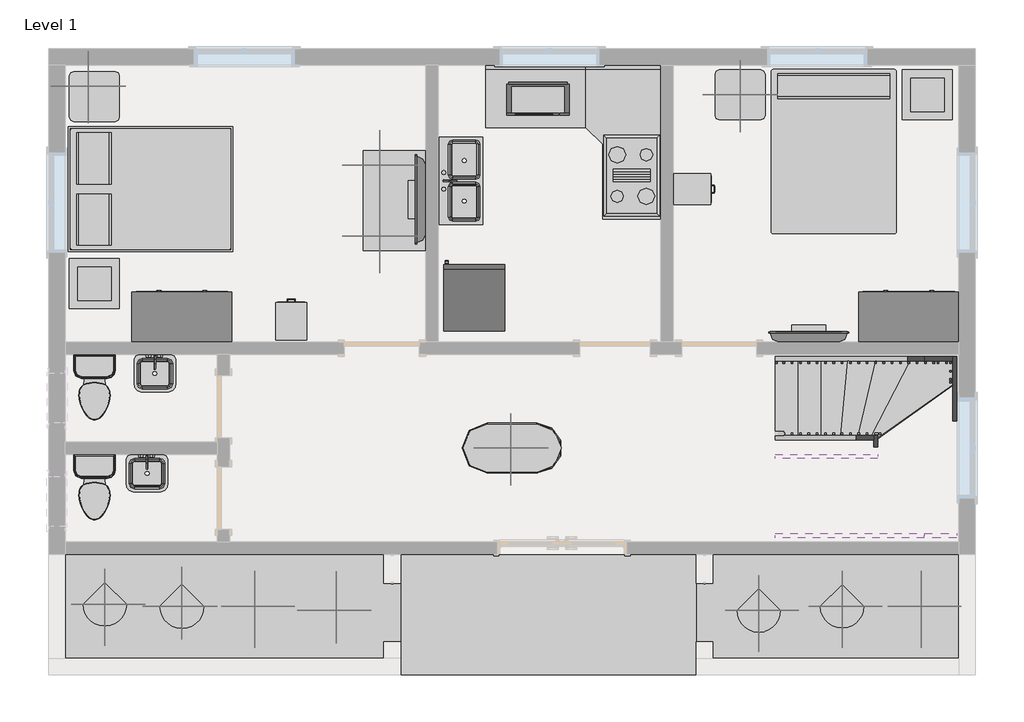
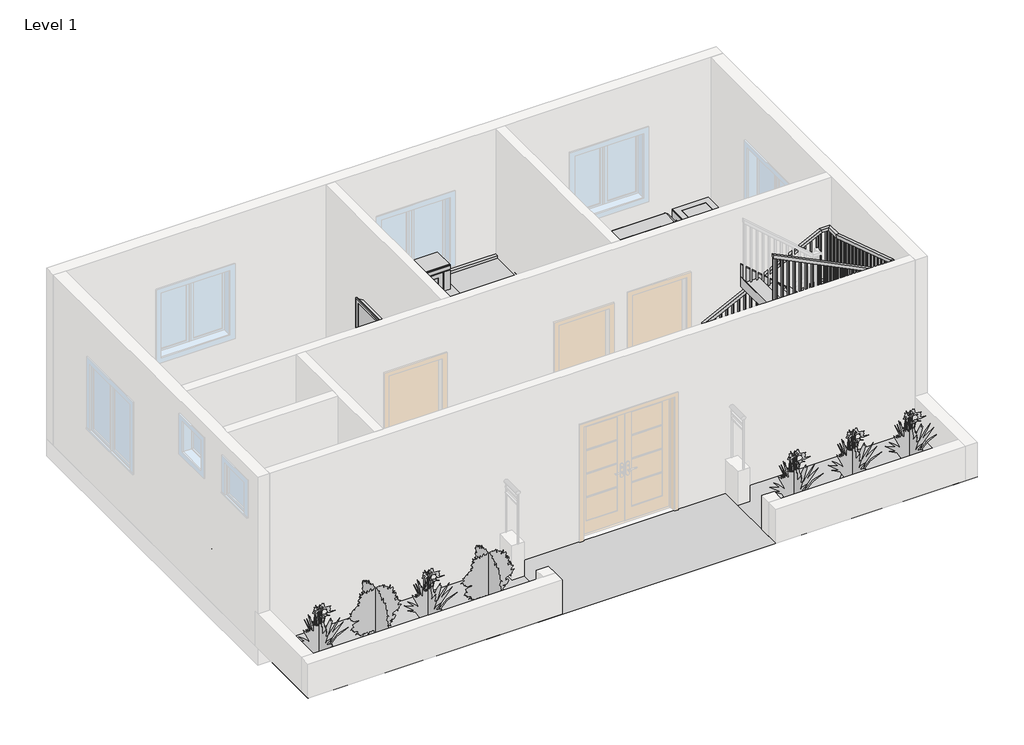
# One storey, part 2 of 2: 15 furniture elements, 12 geographic elements, 8 members, 7 flow terminals, 6 proxies, 1 railing, 1 stair flight.
"""IFC4 building model written with IfcOpenShell, lengths in millimetres."""

from ifc_helpers import new_model, si_unit, frame, origin, place, context, project, spatial, polyline, outline, extrude, faceted_brep, triangles, transform, mapped, element, save
from components import proxy_bb1e6e30, proxy_8a8d5ab2, proxy_a13a33b2, flow_terminal_accce45a, flow_terminal_a53be723, flow_terminal_62a433f7, toilet_domestic_3d_toilet_domestic_3d_f7549cf7, toilet_domestic_3d_toilet_domestic_3d_183bbd19, furniture_1d2926bd, furniture_e1791683, furniture_bb55ed6b, furniture_9fa109b2, furniture_4831bac8, furniture_7a3aaa4f, furniture_b5c51a22, furniture_6551fbda, furniture_31d08a24, furniture_3f969c1c, furniture_5f8511dd, rpc_plant_tropical_55f6ff97, rpc_plant_tropical_agave_1_5_93a2a214, rpc_plant_tropical_jungle_flame_3_9c4808c2, stair_flight_f6c8c564

model = new_model("IFC4")

# Units and contexts
model_context = context("Model", 3, world=origin())
ifc_project = project(units=[si_unit("LENGTHUNIT", "METRE", prefix="MILLI")], contexts=[model_context])

# Site, building, storey
site = spatial("IfcSite", under=ifc_project)
building = spatial("IfcBuilding", under=site)
storey = spatial("IfcBuildingStorey", under=building, Name="Level 1", Elevation=0.0)

# Proxies
placement = place(None, origin())
element("IfcBuildingElementProxy", 1, Name="Building Element Proxy", at=placement, inside=storey, context=model_context, shape_type="Tessellation", body=[
    triangles([(-14311.9113007, 8123.9355194, 0.0), (-14311.9113007, 6650.7353256, 0.0), (-10019.3116882, 8123.9355194, 0.0), (-10019.3116882, 6650.7353256, 0.0)], [[1, 2, 3], [4, 3, 2]], closed=False),
])
element("IfcBuildingElementProxy", 2, Name="Building Element Proxy", at=placement, inside=storey, context=model_context, shape_type="Tessellation", body=[
    triangles([(-10019.3116882, 8123.9355194, 0.0), (-10019.3116882, 6650.7353256, 0.0), (-6412.5120758, 8123.9355194, 0.0), (-6412.5120758, 6650.7353256, 0.0)], [[1, 2, 3], [4, 3, 2]], closed=False),
])
element("IfcBuildingElementProxy", 3, Name="Building Element Proxy", at=placement, inside=storey, context=model_context, shape_type="Tessellation", body=[
    triangles([(-6209.3116882, 8123.9355194, 0.0), (-6412.5120758, 8123.9355194, 0.0), (-6412.5120758, 6650.7353256, 0.0), (-3008.9119789, 8123.9355194, 0.0), (-3008.9119789, 6650.7353256, 0.0)], [[2, 3, 1], [1, 5, 4], [5, 1, 3]], closed=False),
])
proxy_shape = proxy_bb1e6e30(model_context)
element("IfcBuildingElementProxy", 4, Name="Cook Top-4 Unit : 36\" x 20\"", ObjectType="Cook Top-4 Unit : 36\" x 20\"", at=placement, inside=storey, context=model_context, shape_type="MappedRepresentation", body=[
    mapped(proxy_shape, transform((-7199.9118598, 12746.7355643, 0.0), x_axis=(0.0, -1.0000000000000007, 0.0), y_axis=(1.0000000000000007, 0.0, 0.0), z_axis=(0.0, 0.0, 1.0))),
])
proxy_2_shape = proxy_8a8d5ab2(model_context)
element("IfcBuildingElementProxy", 5, Name="Microwave : 30\" x 16\" x 18\"", ObjectType="Microwave : 30\" x 16\" x 18\"", at=placement, inside=storey, context=model_context, shape_type="MappedRepresentation", body=[
    mapped(proxy_2_shape, transform((-8843.2047371, 14039.6160702, 0.0), x_axis=(1.0000000000000022, 0.0, 0.0), y_axis=(0.0, 1.0000000000000022, 0.0), z_axis=(0.0, 0.0, 1.0))),
])
proxy_3_shape = proxy_a13a33b2(model_context)
element("IfcBuildingElementProxy", 6, Name="Refrigerator : 30\" x 32\" RH", ObjectType="Refrigerator : 30\" x 32\" RH", at=placement, inside=storey, context=model_context, shape_type="MappedRepresentation", body=[
    mapped(proxy_3_shape, transform((-9122.3743598, 11240.5865929, 0.0), x_axis=(-1.0000000000000004, 0.0, 0.0), y_axis=(0.0, -1.0000000000000004, 0.0), z_axis=(0.0, 0.0, 1.0))),
])

# Flow terminals
flow_terminal_shape = flow_terminal_accce45a(model_context)
element("IfcFlowTerminal", 7, ObjectType="Floor Drain - Round : 5\" Strainer - 2\" Drain", at=placement, inside=storey, context=model_context, shape_type="MappedRepresentation", body=[
    mapped(flow_terminal_shape, transform((-13626.1118598, 8454.1355643, 0.0), x_axis=(1.0, 0.0, 0.0), y_axis=(0.0, 1.0, 0.0), z_axis=(0.0, 0.0, 1.0))),
])
element("IfcFlowTerminal", 8, ObjectType="Floor Drain - Round : 5\" Strainer - 2\" Drain", at=placement, inside=storey, context=model_context, shape_type="MappedRepresentation", body=[
    mapped(flow_terminal_shape, transform((-13626.1118598, 9647.9355643, 0.0), x_axis=(1.0, 0.0, 0.0), y_axis=(0.0, 1.0, 0.0), z_axis=(0.0, 0.0, 1.0))),
])
flow_terminal_2_shape = flow_terminal_a53be723(model_context)
element("IfcFlowTerminal", 9, ObjectType="Sink Kitchen-Double : 42\" x 21\"", at=placement, inside=storey, context=model_context, shape_type="MappedRepresentation", body=[
    mapped(flow_terminal_2_shape, transform((-9280.3664587, 12667.5463238, 0.0), x_axis=(0.0, 1.0, 0.0), y_axis=(-1.0, 0.0, 0.0), z_axis=(0.0, 0.0, 1.0))),
])
flow_terminal_3_shape = flow_terminal_62a433f7(model_context)
element("IfcFlowTerminal", 10, ObjectType="Sink Vanity-Square : 20\" x 18\"", at=placement, inside=storey, context=model_context, shape_type="MappedRepresentation", body=[
    mapped(flow_terminal_3_shape, transform((-13032.2011003, 10382.1901632, 0.0), x_axis=(1.0, 0.0, 0.0), y_axis=(0.0, 1.0, 0.0), z_axis=(0.0, 0.0, 1.0))),
])
element("IfcFlowTerminal", 11, ObjectType="Sink Vanity-Square : 20\" x 18\"", at=placement, inside=storey, context=model_context, shape_type="MappedRepresentation", body=[
    mapped(flow_terminal_3_shape, transform((-13127.4511003, 9162.9901632, 0.0), x_axis=(1.0, 0.0, 0.0), y_axis=(0.0, 1.0, 0.0), z_axis=(0.0, 0.0, 1.0))),
])
toilet_domestic_3d_toilet_domestic_3d_shape = toilet_domestic_3d_toilet_domestic_3d_f7549cf7(model_context)
toilet_domestic_3d_toilet_domestic_3d_2_shape = toilet_domestic_3d_toilet_domestic_3d_183bbd19(model_context)
element("IfcFlowTerminal", 12, ObjectType="Toilet-Domestic-3D : Toilet-Domestic-3D", at=placement, inside=storey, context=model_context, shape_type="MappedRepresentation", body=[
    mapped(toilet_domestic_3d_toilet_domestic_3d_shape, transform((-13753.1118598, 10067.639537, 0.0), x_axis=(1.0, 0.0, 0.0), y_axis=(0.0, 1.0, 0.0), z_axis=(0.0, 0.0, 1.0))),
    mapped(toilet_domestic_3d_toilet_domestic_3d_2_shape, transform((-13753.1118598, 10067.639537, 0.0), x_axis=(1.0, 0.0, 0.0), y_axis=(0.0, 1.0, 0.0), z_axis=(0.0, 0.0, 1.0))),
])
element("IfcFlowTerminal", 13, ObjectType="Toilet-Domestic-3D : Toilet-Domestic-3D", at=placement, inside=storey, context=model_context, shape_type="MappedRepresentation", body=[
    mapped(toilet_domestic_3d_toilet_domestic_3d_shape, transform((-13753.1118598, 8848.439537, 0.0), x_axis=(1.0, 0.0, 0.0), y_axis=(0.0, 1.0, 0.0), z_axis=(0.0, 0.0, 1.0))),
    mapped(toilet_domestic_3d_toilet_domestic_3d_2_shape, transform((-13753.1118598, 8848.439537, 0.0), x_axis=(1.0, 0.0, 0.0), y_axis=(0.0, 1.0, 0.0), z_axis=(0.0, 0.0, 1.0))),
])

# Furniture
furniture_shape = furniture_1d2926bd(model_context)
element("IfcFurniture", 14, ObjectType="Bed-Box : Queen 60\" x 79\"", at=placement, inside=storey, context=model_context, shape_type="MappedRepresentation", body=[
    mapped(furniture_shape, transform((-13301.741368, 12242.4831053, 0.0), x_axis=(0.0, 1.0000000000000002, 0.0), y_axis=(-1.0000000000000002, 0.0, 0.0), z_axis=(0.0, 0.0, 1.0))),
])
furniture_2_shape = furniture_e1791683(model_context)
element("IfcFurniture", 15, ObjectType="Bed-Standard.0001 : Queen 60\" x 79\"", at=placement, inside=storey, context=model_context, shape_type="MappedRepresentation", body=[
    mapped(furniture_2_shape, transform((-5007.6003844, 13084.4306463, 0.0), x_axis=(1.0000000000000004, 0.0, 0.0), y_axis=(0.0, 1.0000000000000004, 0.0), z_axis=(0.0, 0.0, 1.0))),
])
furniture_3_shape = furniture_bb55ed6b(model_context)
element("IfcFurniture", 16, ObjectType="Cabinet-File 2 Drawer : 15\" x 18\"", at=placement, inside=storey, context=model_context, shape_type="MappedRepresentation", body=[
    mapped(furniture_3_shape, transform((-11480.7083068, 10826.6012642, 0.0), x_axis=(-0.9999999999999998, 0.0, 0.0), y_axis=(0.0, -0.9999999999999998, 0.0), z_axis=(0.0, 0.0, 1.0))),
])
element("IfcFurniture", 17, ObjectType="Cabinet-File 2 Drawer : 15\" x 18\"", at=placement, inside=storey, context=model_context, shape_type="MappedRepresentation", body=[
    mapped(furniture_3_shape, transform((-6605.4461599, 12709.5320114, 0.0), x_axis=(0.0, 1.0000000000000002, 0.0), y_axis=(-1.0000000000000002, 0.0, 0.0), z_axis=(0.0, 0.0, 1.0))),
])
furniture_4_shape = furniture_9fa109b2(model_context)
element("IfcFurniture", 18, ObjectType="Dresser : 48\" x 72\" x 24\"", at=placement, inside=storey, context=model_context, shape_type="MappedRepresentation", body=[
    mapped(furniture_4_shape, transform((-12955.5051196, 10656.3726102, 0.0), x_axis=(-1.0000000000000004, 0.0, 0.0), y_axis=(0.0, -1.0000000000000004, 0.0), z_axis=(0.0, 0.0, 1.0))),
])
element("IfcFurniture", 19, ObjectType="Dresser : 48\" x 72\" x 24\"", at=placement, inside=storey, context=model_context, shape_type="MappedRepresentation", body=[
    mapped(furniture_4_shape, transform((-4090.9051196, 10656.3726102, 0.0), x_axis=(-1.0000000000000004, 0.0, 0.0), y_axis=(0.0, -1.0000000000000004, 0.0), z_axis=(0.0, 0.0, 1.0))),
])
furniture_5_shape = furniture_4831bac8(model_context)
element("IfcFurniture", 20, ObjectType="TV - Flat Screen : 37\"", at=placement, inside=storey, context=model_context, shape_type="MappedRepresentation", body=[
    mapped(furniture_5_shape, transform((-5044.8563739, 10773.274188, 990.6), x_axis=(-1.0000000000000004, 0.0, 0.0), y_axis=(0.0, -1.0000000000000004, 0.0), z_axis=(0.0, 0.0, 1.0))),
])
furniture_6_shape = furniture_7a3aaa4f(model_context)
element("IfcFurniture", 21, ObjectType="TV - Flat Screen : 42\"", at=placement, inside=storey, context=model_context, shape_type="MappedRepresentation", body=[
    mapped(furniture_6_shape, transform((-9773.0504834, 12450.6910502, 1041.4), x_axis=(0.0, -1.0000000000000004, 0.0), y_axis=(1.0000000000000004, 0.0, 0.0), z_axis=(0.0, 0.0, 1.0))),
])
furniture_7_shape = furniture_b5c51a22(model_context)
element("IfcFurniture", 22, ObjectType="Table-Coffee : 24\" x 24\" x 24\"", at=placement, inside=storey, context=model_context, shape_type="MappedRepresentation", body=[
    mapped(furniture_7_shape, transform((-13771.3776265, 11330.7244865, 0.0), x_axis=(1.0, 0.0, 0.0), y_axis=(0.0, 1.0, 0.0), z_axis=(0.0, 0.0, 1.0))),
])
element("IfcFurniture", 23, ObjectType="Table-Coffee : 24\" x 24\" x 24\"", at=placement, inside=storey, context=model_context, shape_type="MappedRepresentation", body=[
    mapped(furniture_7_shape, transform((-3611.3776265, 13635.7744865, 0.0), x_axis=(1.0, 0.0, 0.0), y_axis=(0.0, 1.0, 0.0), z_axis=(0.0, 0.0, 1.0))),
])
furniture_8_shape = furniture_6551fbda(model_context)
element("IfcFurniture", 24, ObjectType="Table-Dining Oval : 36\" x 48\"", at=placement, inside=storey, context=model_context, shape_type="MappedRepresentation", body=[
    mapped(furniture_8_shape, transform((-8258.5921876, 9777.433925, 0.0), x_axis=(1.0, 0.0, 0.0), y_axis=(0.0, 1.0, 0.0), z_axis=(0.0, 0.0, 1.0))),
])
furniture_9_shape = furniture_31d08a24(model_context)
element("IfcFurniture", 25, ObjectType="Table-End : 24\" x 24\"", at=placement, inside=storey, context=model_context, shape_type="MappedRepresentation", body=[
    mapped(furniture_9_shape, transform((-14061.6454901, 13559.5355643, 0.0), x_axis=(1.0, 0.0, 0.0), y_axis=(0.0, 1.0, 0.0), z_axis=(0.0, 0.0, 1.0))),
])
element("IfcFurniture", 26, ObjectType="Table-End : 24\" x 24\"", at=placement, inside=storey, context=model_context, shape_type="MappedRepresentation", body=[
    mapped(furniture_9_shape, transform((-6187.6454901, 13578.5855643, 0.0), x_axis=(1.0, 0.0, 0.0), y_axis=(0.0, 1.0, 0.0), z_axis=(0.0, 0.0, 1.0))),
])
furniture_10_shape = furniture_3f969c1c(model_context)
element("IfcFurniture", 27, ObjectType="Table-Rectangular : 72\" x 30\"", at=placement, inside=storey, context=model_context, shape_type="MappedRepresentation", body=[
    mapped(furniture_10_shape, transform((-10095.5118598, 12441.9355643, 0.0), x_axis=(0.0, 1.0000000000000002, 0.0), y_axis=(-1.0000000000000002, 0.0, 0.0), z_axis=(0.0, 0.0, 1.0))),
])
furniture_11_shape = furniture_5f8511dd(model_context)
element("IfcFurniture", 28, ObjectType="Work Station Cubicle : 96\" x 96\"", at=placement, inside=storey, context=model_context, shape_type="MappedRepresentation", body=[
    mapped(furniture_11_shape, transform((-6298.4888522, 13961.2038121, 0.0), x_axis=(0.0, -1.0000000000000013, 0.0), y_axis=(1.0000000000000013, 0.0, 0.0), z_axis=(0.0, 0.0, 1.0))),
])

# Geographic elements
rpc_plant_tropical_shape = rpc_plant_tropical_55f6ff97(model_context)
element("IfcGeographicElement", 29, ObjectType="RPC Plant - Tropical", at=placement, inside=storey, context=model_context, shape_type="MappedRepresentation", body=[
    mapped(rpc_plant_tropical_shape, transform((-13626.1118598, 7514.3355643, 0.0), x_axis=(1.0, 0.0, 0.0), y_axis=(0.0, 1.0, 0.0), z_axis=(0.0, 0.0, 1.0))),
])
element("IfcGeographicElement", 30, ObjectType="RPC Plant - Tropical", at=placement, inside=storey, context=model_context, shape_type="MappedRepresentation", body=[
    mapped(rpc_plant_tropical_shape, transform((-11797.3118598, 7488.9355643, 0.0), x_axis=(1.0, 0.0, 0.0), y_axis=(0.0, 1.0, 0.0), z_axis=(0.0, 0.0, 1.0))),
])
element("IfcGeographicElement", 31, ObjectType="RPC Plant - Tropical", at=placement, inside=storey, context=model_context, shape_type="MappedRepresentation", body=[
    mapped(rpc_plant_tropical_shape, transform((-5650.5118598, 7438.1355643, 0.0), x_axis=(1.0, 0.0, 0.0), y_axis=(0.0, 1.0, 0.0), z_axis=(0.0, 0.0, 1.0))),
])
element("IfcGeographicElement", 32, ObjectType="RPC Plant - Tropical", at=placement, inside=storey, context=model_context, shape_type="MappedRepresentation", body=[
    mapped(rpc_plant_tropical_shape, transform((-3669.3118598, 7488.9355643, 0.0), x_axis=(1.0, 0.0, 0.0), y_axis=(0.0, 1.0, 0.0), z_axis=(0.0, 0.0, 1.0))),
])
element("IfcGeographicElement", 33, ObjectType="RPC Plant - Tropical", at=placement, inside=storey, context=model_context, shape_type="MappedRepresentation", body=[
    mapped(rpc_plant_tropical_shape, transform((-4634.5118598, 7488.9355643, 0.0), x_axis=(1.0, 0.0, 0.0), y_axis=(0.0, 1.0, 0.0), z_axis=(0.0, 0.0, 1.0))),
])
rpc_plant_tropical_agave_1_5_shape = rpc_plant_tropical_agave_1_5_93a2a214(model_context)
element("IfcGeographicElement", 34, ObjectType="RPC Plant - Tropical : Agave - 1.5'", at=placement, inside=storey, context=model_context, shape_type="MappedRepresentation", body=[
    mapped(rpc_plant_tropical_agave_1_5_shape, transform((-13829.3118598, 13838.9355643, 609.6), x_axis=(1.0, 0.0, 0.0), y_axis=(0.0, 1.0, 0.0), z_axis=(0.0, 0.0, 1.0))),
])
element("IfcGeographicElement", 35, ObjectType="RPC Plant - Tropical : Agave - 1.5'", at=placement, inside=storey, context=model_context, shape_type="MappedRepresentation", body=[
    mapped(rpc_plant_tropical_agave_1_5_shape, transform((-10273.3118598, 12010.1355643, 660.4), x_axis=(1.0, 0.0, 0.0), y_axis=(0.0, 1.0, 0.0), z_axis=(0.0, 0.0, 1.0))),
])
element("IfcGeographicElement", 36, ObjectType="RPC Plant - Tropical : Agave - 1.5'", at=placement, inside=storey, context=model_context, shape_type="MappedRepresentation", body=[
    mapped(rpc_plant_tropical_agave_1_5_shape, transform((-10273.3118598, 12873.7355643, 660.4), x_axis=(1.0, 0.0, 0.0), y_axis=(0.0, 1.0, 0.0), z_axis=(0.0, 0.0, 1.0))),
])
element("IfcGeographicElement", 37, ObjectType="RPC Plant - Tropical : Agave - 1.5'", at=placement, inside=storey, context=model_context, shape_type="MappedRepresentation", body=[
    mapped(rpc_plant_tropical_agave_1_5_shape, transform((-5879.1118598, 13730.9855643, 609.6), x_axis=(1.0, 0.0, 0.0), y_axis=(0.0, 1.0, 0.0), z_axis=(0.0, 0.0, 1.0))),
])
element("IfcGeographicElement", 38, ObjectType="RPC Plant - Tropical : Agave - 1.5'", at=placement, inside=storey, context=model_context, shape_type="MappedRepresentation", body=[
    mapped(rpc_plant_tropical_agave_1_5_shape, transform((-8673.1118598, 9419.3355643, 736.6), x_axis=(1.0, 0.0, 0.0), y_axis=(0.0, 1.0, 0.0), z_axis=(0.0, 0.0, 1.0))),
])
rpc_plant_tropical_jungle_flame_3_shape = rpc_plant_tropical_jungle_flame_3_9c4808c2(model_context)
element("IfcGeographicElement", 39, ObjectType="RPC Plant - Tropical : Jungle Flame - 3'", at=placement, inside=storey, context=model_context, shape_type="MappedRepresentation", body=[
    mapped(rpc_plant_tropical_jungle_flame_3_shape, transform((-12686.3118598, 7488.9355643, 0.0), x_axis=(1.0, 0.0, 0.0), y_axis=(0.0, 1.0, 0.0), z_axis=(0.0, 0.0, 1.0))),
])
element("IfcGeographicElement", 40, ObjectType="RPC Plant - Tropical : Jungle Flame - 3'", at=placement, inside=storey, context=model_context, shape_type="MappedRepresentation", body=[
    mapped(rpc_plant_tropical_jungle_flame_3_shape, transform((-10806.7118598, 7438.1355643, 0.0), x_axis=(1.0, 0.0, 0.0), y_axis=(0.0, 1.0, 0.0), z_axis=(0.0, 0.0, 1.0))),
])

# Members
element("IfcMember", 41, ObjectType="Stringer - 2\" Width", at=placement, inside=storey, context=model_context, shape_type="SweptSolid", body=[
    extrude(outline(polyline([(402.7316435, -5447.3118598), (62.3947048, -5447.3118598), (963.623715, -3633.1160297), (1303.9606537, -3633.1160297), (402.7316435, -5447.3118598)])), frame((0.0, 10486.1355643, 0.0), z_axis=(0.0, 1.0, 0.0), x_axis=(0.0, 0.0, 1.0)), (0.0, 0.0, 1.0), 50.8),
])
element("IfcMember", 42, ObjectType="Stringer - 2\" Width", at=placement, inside=storey, context=model_context, shape_type="SweptSolid", body=[
    extrude(outline(polyline([(-3633.1160297, 10486.1355643), (-3633.1160297, 10536.9355643), (-3284.5801679, 10536.9355643), (-3284.5801679, 10486.1355643), (-3633.1160297, 10486.1355643)])), frame((0.0, 0.0, 963.623715), z_axis=(0.0, 0.0, 1.0), x_axis=(1.0, 0.0, 0.0)), (0.0, 0.0, 1.0), 340.3369387),
])
element("IfcMember", 43, ObjectType="Stringer - 2\" Width", at=placement, inside=storey, context=model_context, shape_type="SweptSolid", body=[
    extrude(outline(polyline([(10536.9355643, 1287.6602296), (10536.9355643, 999.1606537), (10375.3852872, 999.1606537), (8377.9355643, 1640.0913157), (8377.9355643, 1969.9972697), (8410.4435544, 1969.9972697), (10536.9355643, 1287.6602296)])), frame((-3284.5801679, 0.0, 0.0), z_axis=(1.0, 0.0, 0.0), x_axis=(0.0, 1.0, 0.0)), (0.0, 0.0, 1.0), 50.8),
])
element("IfcMember", 44, ObjectType="Stringer - 2\" Width", at=placement, inside=storey, context=model_context, shape_type="SweptSolid", body=[
    extrude(outline(polyline([(-3233.7801679, 8377.9355643), (-3233.7801679, 8327.1355643), (-3633.1160297, 8327.1355643), (-3633.1160297, 8377.9355643), (-3233.7801679, 8377.9355643)])), frame((0.0, 0.0, 1649.8904473), z_axis=(0.0, 0.0, 1.0), x_axis=(1.0, 0.0, 0.0)), (0.0, 0.0, 1.0), 320.1068224),
])
element("IfcMember", 45, ObjectType="Stringer - 2\" Width", at=placement, inside=storey, context=model_context, shape_type="SweptSolid", body=[
    extrude(outline(polyline([(1649.8904473, -3633.1160297), (1969.9972697, -3633.1160297), (2871.2262799, -5447.3118598), (2551.1194575, -5447.3118598), (1649.8904473, -3633.1160297)])), frame((0.0, 8327.1355643, 0.0), z_axis=(0.0, 1.0, 0.0), x_axis=(0.0, 0.0, 1.0)), (0.0, 0.0, 1.0), 50.8),
])
element("IfcMember", 46, ObjectType="Stringer - 2\" Width", at=placement, inside=storey, context=model_context, shape_type="SweptSolid", body=[
    extrude(outline(polyline([(336.1105785, -5447.3118598), (0.0, -5447.3118598), (0.0, -5368.4508455), (979.8041326, -4249.7801679), (1384.986288, -4249.7801679), (336.1105785, -5447.3118598)])), frame((0.0, 9520.9355643, 0.0), z_axis=(0.0, 1.0, 0.0), x_axis=(0.0, 0.0, 1.0)), (0.0, 0.0, 1.0), 50.8),
])
element("IfcMember", 47, ObjectType="Stringer - 2\" Width", at=placement, inside=storey, context=model_context, shape_type="SweptSolid", body=[
    extrude(outline(polyline([(9571.7355643, 1573.2682978), (9571.7355643, 1024.2980583), (9539.9901117, 1024.2980583), (9343.1355643, 1360.465107), (9343.1355643, 1933.5074587), (9360.7847373, 1933.5074587), (9571.7355643, 1573.2682978)])), frame((-4249.7801679, 0.0, 0.0), z_axis=(1.0, 0.0, 0.0), x_axis=(0.0, 1.0, 0.0)), (0.0, 0.0, 1.0), 50.8),
])
element("IfcMember", 48, ObjectType="Stringer - 2\" Width", at=placement, inside=storey, context=model_context, shape_type="SweptSolid", body=[
    extrude(outline(polyline([(1528.3253033, -4198.9801679), (1933.5074587, -4198.9801679), (3026.8770938, -5447.3118598), (2621.6949384, -5447.3118598), (1528.3253033, -4198.9801679)])), frame((0.0, 9292.3355643, 0.0), z_axis=(0.0, 1.0, 0.0), x_axis=(0.0, 0.0, 1.0)), (0.0, 0.0, 1.0), 50.8),
])

# Railing
element("IfcRailing", 49, ObjectType="Handrail - Rectangular", at=placement, inside=storey, context=model_context, shape_type="SolidModel", body=[
    faceted_brep([(-5447.3118598, 10486.1355643, 1283.6038561), (-5447.3118598, 10486.1355643, 1226.881033), (-5447.3118598, 10435.3355643, 1226.881033), (-5447.3118598, 10435.3355643, 1283.6038561), (-3463.3448117, 10486.1355643, 2269.1692672), (-3451.4220252, 10486.1355643, 2218.3692672), (-3451.4220252, 10435.3355643, 2218.3692672), (-3463.3448117, 10435.3355643, 2269.1692672), (-3284.5801679, 10486.1355643, 2269.1692672), (-3284.5801679, 10486.1355643, 2218.3692672), (-3335.3801679, 10435.3355643, 2218.3692672), (-3335.3801679, 10435.3355643, 2269.1692672), (-3284.5801679, 10223.302577, 2269.1692672), (-3284.5801679, 10215.3520009, 2218.3692672), (-3335.3801679, 10215.3520009, 2218.3692672), (-3335.3801679, 10223.302577, 2269.1692672), (-3284.5801679, 8640.7685517, 2776.9640661), (-3284.5801679, 8632.8179755, 2726.1640661), (-3335.3801679, 8632.8179755, 2726.1640661), (-3335.3801679, 8640.7685517, 2776.9640661), (-3284.5801679, 8377.9355643, 2776.9640661), (-3284.5801679, 8377.9355643, 2726.1640661), (-3335.3801679, 8428.7355643, 2726.1640661), (-3335.3801679, 8428.7355643, 2776.9640661), (-3463.3448117, 8377.9355643, 2776.9640661), (-3475.2675981, 8377.9355643, 2726.1640661), (-3475.2675981, 8428.7355643, 2726.1640661), (-3463.3448117, 8428.7355643, 2776.9640661), (-5447.3118598, 8377.9355643, 3762.5294772), (-5447.3118598, 8428.7355643, 3762.5294772), (-5447.3118598, 8428.7355643, 3705.8066541), (-5447.3118598, 8377.9355643, 3705.8066541)], [[[0, 1, 2, 3]], [[1, 0, 4, 5]], [[2, 1, 5, 6]], [[3, 2, 6, 7]], [[0, 3, 7, 4]], [[5, 4, 8, 9]], [[6, 5, 9, 10]], [[7, 6, 10, 11]], [[4, 7, 11, 8]], [[9, 8, 12, 13]], [[10, 9, 13, 14]], [[11, 10, 14, 15]], [[8, 11, 15, 12]], [[13, 12, 16, 17]], [[14, 13, 17, 18]], [[15, 14, 18, 19]], [[12, 15, 19, 16]], [[17, 16, 20, 21]], [[18, 17, 21, 22]], [[19, 18, 22, 23]], [[16, 19, 23, 20]], [[21, 20, 24, 25]], [[22, 21, 25, 26]], [[23, 22, 26, 27]], [[20, 23, 27, 24]], [[28, 29, 30, 31]], [[25, 24, 28, 31]], [[26, 25, 31, 30]], [[27, 26, 30, 29]], [[24, 27, 29, 28]]]),
    extrude(outline(polyline([(3683.9281056, -5403.2698117), (2709.3333333, -5403.2698117), (2709.3333333, -5384.2198117), (3674.4647321, -5384.2198117), (3683.9281056, -5403.2698117)])), frame((0.0, 8393.8105643, 0.0), z_axis=(0.0, 1.0, 0.0), x_axis=(0.0, 0.0, 1.0)), (0.0, 0.0, 1.0), 19.05),
    extrude(outline(polyline([(3633.4567805, -5301.6698117), (2709.3333333, -5301.6698117), (2709.3333333, -5282.6198117), (3623.9934071, -5282.6198117), (3633.4567805, -5301.6698117)])), frame((0.0, 8393.8105643, 0.0), z_axis=(0.0, 1.0, 0.0), x_axis=(0.0, 0.0, 1.0)), (0.0, 0.0, 1.0), 19.05),
    extrude(outline(polyline([(3582.9854555, -5200.0698117), (2709.3333333, -5200.0698117), (2709.3333333, -5181.0198117), (3573.5220821, -5181.0198117), (3582.9854555, -5200.0698117)])), frame((0.0, 8393.8105643, 0.0), z_axis=(0.0, 1.0, 0.0), x_axis=(0.0, 0.0, 1.0)), (0.0, 0.0, 1.0), 19.05),
    extrude(outline(polyline([(3532.5141305, -5098.4698117), (2540.0, -5098.4698117), (2540.0, -5079.4198117), (3523.050757, -5079.4198117), (3532.5141305, -5098.4698117)])), frame((0.0, 8393.8105643, 0.0), z_axis=(0.0, 1.0, 0.0), x_axis=(0.0, 0.0, 1.0)), (0.0, 0.0, 1.0), 19.05),
    extrude(outline(polyline([(3482.0428054, -4996.8698117), (2540.0, -4996.8698117), (2540.0, -4977.8198117), (3472.579432, -4977.8198117), (3482.0428054, -4996.8698117)])), frame((0.0, 8393.8105643, 0.0), z_axis=(0.0, 1.0, 0.0), x_axis=(0.0, 0.0, 1.0)), (0.0, 0.0, 1.0), 19.05),
    extrude(outline(polyline([(3431.5714804, -4895.2698117), (2370.6666667, -4895.2698117), (2370.6666667, -4876.2198117), (3422.1081069, -4876.2198117), (3431.5714804, -4895.2698117)])), frame((0.0, 8393.8105643, 0.0), z_axis=(0.0, 1.0, 0.0), x_axis=(0.0, 0.0, 1.0)), (0.0, 0.0, 1.0), 19.05),
    extrude(outline(polyline([(3381.1001553, -4793.6698117), (2370.6666667, -4793.6698117), (2370.6666667, -4774.6198117), (3371.6367819, -4774.6198117), (3381.1001553, -4793.6698117)])), frame((0.0, 8393.8105643, 0.0), z_axis=(0.0, 1.0, 0.0), x_axis=(0.0, 0.0, 1.0)), (0.0, 0.0, 1.0), 19.05),
    extrude(outline(polyline([(3330.6288303, -4692.0698117), (2370.6666667, -4692.0698117), (2370.6666667, -4673.0198117), (3321.1654568, -4673.0198117), (3330.6288303, -4692.0698117)])), frame((0.0, 8393.8105643, 0.0), z_axis=(0.0, 1.0, 0.0), x_axis=(0.0, 0.0, 1.0)), (0.0, 0.0, 1.0), 19.05),
    extrude(outline(polyline([(3280.1575052, -4590.4698117), (2370.6666667, -4590.4698117), (2370.6666667, -4571.4198117), (3270.6941318, -4571.4198117), (3280.1575052, -4590.4698117)])), frame((0.0, 8393.8105643, 0.0), z_axis=(0.0, 1.0, 0.0), x_axis=(0.0, 0.0, 1.0)), (0.0, 0.0, 1.0), 19.05),
    extrude(outline(polyline([(3229.6861802, -4488.8698117), (2201.3333333, -4488.8698117), (2201.3333333, -4469.8198117), (3220.2228067, -4469.8198117), (3229.6861802, -4488.8698117)])), frame((0.0, 8393.8105643, 0.0), z_axis=(0.0, 1.0, 0.0), x_axis=(0.0, 0.0, 1.0)), (0.0, 0.0, 1.0), 19.05),
    extrude(outline(polyline([(3179.2148551, -4387.2698117), (2201.3333333, -4387.2698117), (2201.3333333, -4368.2198117), (3169.7514817, -4368.2198117), (3179.2148551, -4387.2698117)])), frame((0.0, 8393.8105643, 0.0), z_axis=(0.0, 1.0, 0.0), x_axis=(0.0, 0.0, 1.0)), (0.0, 0.0, 1.0), 19.05),
    extrude(outline(polyline([(3128.7435301, -4285.6698117), (2201.3333333, -4285.6698117), (2201.3333333, -4266.6198117), (3119.2801567, -4266.6198117), (3128.7435301, -4285.6698117)])), frame((0.0, 8393.8105643, 0.0), z_axis=(0.0, 1.0, 0.0), x_axis=(0.0, 0.0, 1.0)), (0.0, 0.0, 1.0), 19.05),
    extrude(outline(polyline([(3078.2722051, -4184.0698117), (2032.0, -4184.0698117), (2032.0, -4165.0198117), (3068.8088316, -4165.0198117), (3078.2722051, -4184.0698117)])), frame((0.0, 8393.8105643, 0.0), z_axis=(0.0, 1.0, 0.0), x_axis=(0.0, 0.0, 1.0)), (0.0, 0.0, 1.0), 19.05),
    extrude(outline(polyline([(3027.80088, -4082.4698117), (2032.0, -4082.4698117), (2032.0, -4063.4198117), (3018.3375066, -4063.4198117), (3027.80088, -4082.4698117)])), frame((0.0, 8393.8105643, 0.0), z_axis=(0.0, 1.0, 0.0), x_axis=(0.0, 0.0, 1.0)), (0.0, 0.0, 1.0), 19.05),
    extrude(outline(polyline([(2977.329555, -3980.8698117), (2032.0, -3980.8698117), (2032.0, -3961.8198117), (2967.8661815, -3961.8198117), (2977.329555, -3980.8698117)])), frame((0.0, 8393.8105643, 0.0), z_axis=(0.0, 1.0, 0.0), x_axis=(0.0, 0.0, 1.0)), (0.0, 0.0, 1.0), 19.05),
    extrude(outline(polyline([(2926.8582299, -3879.2698117), (2032.0, -3879.2698117), (2032.0, -3860.2198117), (2917.3948565, -3860.2198117), (2926.8582299, -3879.2698117)])), frame((0.0, 8393.8105643, 0.0), z_axis=(0.0, 1.0, 0.0), x_axis=(0.0, 0.0, 1.0)), (0.0, 0.0, 1.0), 19.05),
    extrude(outline(polyline([(2876.3869049, -3777.6698117), (1862.6666667, -3777.6698117), (1862.6666667, -3758.6198117), (2866.9235314, -3758.6198117), (2876.3869049, -3777.6698117)])), frame((0.0, 8393.8105643, 0.0), z_axis=(0.0, 1.0, 0.0), x_axis=(0.0, 0.0, 1.0)), (0.0, 0.0, 1.0), 19.05),
    extrude(outline(polyline([(2825.9155798, -3676.0698117), (1862.6666667, -3676.0698117), (1862.6666667, -3657.0198117), (2816.4522064, -3657.0198117), (2825.9155798, -3676.0698117)])), frame((0.0, 8393.8105643, 0.0), z_axis=(0.0, 1.0, 0.0), x_axis=(0.0, 0.0, 1.0)), (0.0, 0.0, 1.0), 19.05),
    extrude(outline(polyline([(2775.4442548, -3574.4698117), (1862.6666667, -3574.4698117), (1862.6666667, -3555.4198117), (2765.9808813, -3555.4198117), (2775.4442548, -3574.4698117)])), frame((0.0, 8393.8105643, 0.0), z_axis=(0.0, 1.0, 0.0), x_axis=(0.0, 0.0, 1.0)), (0.0, 0.0, 1.0), 19.05),
    extrude(outline(polyline([(-3402.0551679, 8393.8105643), (-3421.1051679, 8393.8105643), (-3421.1051679, 8412.8605643), (-3402.0551679, 8412.8605643), (-3402.0551679, 8393.8105643)])), frame((0.0, 0.0, 1862.6666667), z_axis=(0.0, 0.0, 1.0), x_axis=(1.0, 0.0, 0.0)), (0.0, 0.0, 1.0), 863.4973995),
    extrude(outline(polyline([(-3300.4551679, 8447.0935517), (-3300.4551679, 8428.0435517), (-3319.5051679, 8428.0435517), (-3319.5051679, 8447.0935517), (-3300.4551679, 8447.0935517)])), frame((0.0, 0.0, 1862.6666667), z_axis=(0.0, 0.0, 1.0), x_axis=(1.0, 0.0, 0.0)), (0.0, 0.0, 1.0), 863.4973995),
    extrude(outline(polyline([(-3300.4551679, 8548.6935517), (-3300.4551679, 8529.6435517), (-3319.5051679, 8529.6435517), (-3319.5051679, 8548.6935517), (-3300.4551679, 8548.6935517)])), frame((0.0, 0.0, 1862.6666667), z_axis=(0.0, 0.0, 1.0), x_axis=(1.0, 0.0, 0.0)), (0.0, 0.0, 1.0), 863.4973995),
    extrude(outline(polyline([(8708.827577, 2701.774524), (8708.827577, 1693.3333333), (8689.777577, 1693.3333333), (8689.777577, 2707.887183), (8708.827577, 2701.774524)])), frame((-3319.5051679, 0.0, 0.0), z_axis=(1.0, 0.0, 0.0), x_axis=(0.0, 1.0, 0.0)), (0.0, 0.0, 1.0), 19.05),
    extrude(outline(polyline([(8810.427577, 2669.1736758), (8810.427577, 1693.3333333), (8791.377577, 1693.3333333), (8791.377577, 2675.2863348), (8810.427577, 2669.1736758)])), frame((-3319.5051679, 0.0, 0.0), z_axis=(1.0, 0.0, 0.0), x_axis=(0.0, 1.0, 0.0)), (0.0, 0.0, 1.0), 19.05),
    extrude(outline(polyline([(8912.027577, 2636.5728276), (8912.027577, 1693.3333333), (8892.977577, 1693.3333333), (8892.977577, 2642.6854866), (8912.027577, 2636.5728276)])), frame((-3319.5051679, 0.0, 0.0), z_axis=(1.0, 0.0, 0.0), x_axis=(0.0, 1.0, 0.0)), (0.0, 0.0, 1.0), 19.05),
    extrude(outline(polyline([(9013.627577, 2603.9719793), (9013.627577, 1693.3333333), (8994.577577, 1693.3333333), (8994.577577, 2610.0846384), (9013.627577, 2603.9719793)])), frame((-3319.5051679, 0.0, 0.0), z_axis=(1.0, 0.0, 0.0), x_axis=(0.0, 1.0, 0.0)), (0.0, 0.0, 1.0), 19.05),
    extrude(outline(polyline([(9115.227577, 2571.3711311), (9115.227577, 1693.3333333), (9096.177577, 1693.3333333), (9096.177577, 2577.4837901), (9115.227577, 2571.3711311)])), frame((-3319.5051679, 0.0, 0.0), z_axis=(1.0, 0.0, 0.0), x_axis=(0.0, 1.0, 0.0)), (0.0, 0.0, 1.0), 19.05),
    extrude(outline(polyline([(9216.827577, 2538.6676823), (9216.827577, 1680.7777495), (9197.777577, 1680.7777495), (9197.777577, 2544.7803414), (9216.827577, 2538.6676823)])), frame((-3319.5051679, 0.0, 0.0), z_axis=(1.0, 0.0, 0.0), x_axis=(0.0, 1.0, 0.0)), (0.0, 0.0, 1.0), 19.05),
    extrude(outline(polyline([(9318.427577, 2506.1694346), (9318.427577, 1524.0), (9299.377577, 1524.0), (9299.377577, 2512.2820937), (9318.427577, 2506.1694346)])), frame((-3319.5051679, 0.0, 0.0), z_axis=(1.0, 0.0, 0.0), x_axis=(0.0, 1.0, 0.0)), (0.0, 0.0, 1.0), 19.05),
    extrude(outline(polyline([(9420.027577, 2473.5685864), (9420.027577, 1524.0), (9400.977577, 1524.0), (9400.977577, 2479.6812455), (9420.027577, 2473.5685864)])), frame((-3319.5051679, 0.0, 0.0), z_axis=(1.0, 0.0, 0.0), x_axis=(0.0, 1.0, 0.0)), (0.0, 0.0, 1.0), 19.05),
    extrude(outline(polyline([(9521.627577, 2440.9677382), (9521.627577, 1524.0), (9502.577577, 1524.0), (9502.577577, 2447.0803972), (9521.627577, 2440.9677382)])), frame((-3319.5051679, 0.0, 0.0), z_axis=(1.0, 0.0, 0.0), x_axis=(0.0, 1.0, 0.0)), (0.0, 0.0, 1.0), 19.05),
    extrude(outline(polyline([(9623.227577, 2408.36689), (9623.227577, 1524.0), (9604.177577, 1524.0), (9604.177577, 2414.479549), (9623.227577, 2408.36689)])), frame((-3319.5051679, 0.0, 0.0), z_axis=(1.0, 0.0, 0.0), x_axis=(0.0, 1.0, 0.0)), (0.0, 0.0, 1.0), 19.05),
    extrude(outline(polyline([(9724.827577, 2375.7660417), (9724.827577, 1354.6666667), (9705.777577, 1354.6666667), (9705.777577, 2381.8787008), (9724.827577, 2375.7660417)])), frame((-3319.5051679, 0.0, 0.0), z_axis=(1.0, 0.0, 0.0), x_axis=(0.0, 1.0, 0.0)), (0.0, 0.0, 1.0), 19.05),
    extrude(outline(polyline([(9826.427577, 2343.1651935), (9826.427577, 1354.6666667), (9807.377577, 1354.6666667), (9807.377577, 2349.2778526), (9826.427577, 2343.1651935)])), frame((-3319.5051679, 0.0, 0.0), z_axis=(1.0, 0.0, 0.0), x_axis=(0.0, 1.0, 0.0)), (0.0, 0.0, 1.0), 19.05),
    extrude(outline(polyline([(9928.027577, 2310.5643453), (9928.027577, 1354.6666667), (9908.977577, 1354.6666667), (9908.977577, 2316.6770043), (9928.027577, 2310.5643453)])), frame((-3319.5051679, 0.0, 0.0), z_axis=(1.0, 0.0, 0.0), x_axis=(0.0, 1.0, 0.0)), (0.0, 0.0, 1.0), 19.05),
    extrude(outline(polyline([(10029.627577, 2277.9634971), (10029.627577, 1354.6666667), (10010.577577, 1354.6666667), (10010.577577, 2284.0761561), (10029.627577, 2277.9634971)])), frame((-3319.5051679, 0.0, 0.0), z_axis=(1.0, 0.0, 0.0), x_axis=(0.0, 1.0, 0.0)), (0.0, 0.0, 1.0), 19.05),
    extrude(outline(polyline([(10131.227577, 2245.3626488), (10131.227577, 1354.6666667), (10112.177577, 1354.6666667), (10112.177577, 2251.4753079), (10131.227577, 2245.3626488)])), frame((-3319.5051679, 0.0, 0.0), z_axis=(1.0, 0.0, 0.0), x_axis=(0.0, 1.0, 0.0)), (0.0, 0.0, 1.0), 19.05),
    extrude(outline(polyline([(-3300.4551679, 10267.0605643), (-3300.4551679, 10248.0105643), (-3319.5051679, 10248.0105643), (-3319.5051679, 10267.0605643), (-3300.4551679, 10267.0605643)])), frame((0.0, 0.0, 1185.3333333), z_axis=(0.0, 0.0, 1.0), x_axis=(1.0, 0.0, 0.0)), (0.0, 0.0, 1.0), 1033.0359339),
    extrude(outline(polyline([(-3300.4551679, 10368.6605643), (-3300.4551679, 10349.6105643), (-3319.5051679, 10349.6105643), (-3319.5051679, 10368.6605643), (-3300.4551679, 10368.6605643)])), frame((0.0, 0.0, 1185.3333333), z_axis=(0.0, 0.0, 1.0), x_axis=(1.0, 0.0, 0.0)), (0.0, 0.0, 1.0), 1033.0359339),
    extrude(outline(polyline([(-3371.2698117, 10470.2605643), (-3352.2198117, 10470.2605643), (-3352.2198117, 10451.2105643), (-3371.2698117, 10451.2105643), (-3371.2698117, 10470.2605643)])), frame((0.0, 0.0, 1185.3333333), z_axis=(0.0, 0.0, 1.0), x_axis=(1.0, 0.0, 0.0)), (0.0, 0.0, 1.0), 1033.0359339),
    extrude(outline(polyline([(2181.1045221, -3526.4368598), (1185.3333333, -3526.4368598), (1185.3333333, -3507.3868598), (2190.5678956, -3507.3868598), (2181.1045221, -3526.4368598)])), frame((0.0, 10451.2105643, 0.0), z_axis=(0.0, 1.0, 0.0), x_axis=(0.0, 0.0, 1.0)), (0.0, 0.0, 1.0), 19.05),
    extrude(outline(polyline([(2130.6331971, -3628.0368598), (1185.3333333, -3628.0368598), (1185.3333333, -3608.9868598), (2140.0965705, -3608.9868598), (2130.6331971, -3628.0368598)])), frame((0.0, 10451.2105643, 0.0), z_axis=(0.0, 1.0, 0.0), x_axis=(0.0, 0.0, 1.0)), (0.0, 0.0, 1.0), 19.05),
    extrude(outline(polyline([(2080.161872, -3729.6368598), (1185.3333333, -3729.6368598), (1185.3333333, -3710.5868598), (2089.6252455, -3710.5868598), (2080.161872, -3729.6368598)])), frame((0.0, 10451.2105643, 0.0), z_axis=(0.0, 1.0, 0.0), x_axis=(0.0, 0.0, 1.0)), (0.0, 0.0, 1.0), 19.05),
    extrude(outline(polyline([(2029.690547, -3831.2368598), (1016.0, -3831.2368598), (1016.0, -3812.1868598), (2039.1539204, -3812.1868598), (2029.690547, -3831.2368598)])), frame((0.0, 10451.2105643, 0.0), z_axis=(0.0, 1.0, 0.0), x_axis=(0.0, 0.0, 1.0)), (0.0, 0.0, 1.0), 19.05),
    extrude(outline(polyline([(1979.2192219, -3932.8368598), (1016.0, -3932.8368598), (1016.0, -3913.7868598), (1988.6825954, -3913.7868598), (1979.2192219, -3932.8368598)])), frame((0.0, 10451.2105643, 0.0), z_axis=(0.0, 1.0, 0.0), x_axis=(0.0, 0.0, 1.0)), (0.0, 0.0, 1.0), 19.05),
    extrude(outline(polyline([(1928.7478969, -4034.4368598), (1016.0, -4034.4368598), (1016.0, -4015.3868598), (1938.2112704, -4015.3868598), (1928.7478969, -4034.4368598)])), frame((0.0, 10451.2105643, 0.0), z_axis=(0.0, 1.0, 0.0), x_axis=(0.0, 0.0, 1.0)), (0.0, 0.0, 1.0), 19.05),
    extrude(outline(polyline([(1878.2765719, -4136.0368598), (1016.0, -4136.0368598), (1016.0, -4116.9868598), (1887.7399453, -4116.9868598), (1878.2765719, -4136.0368598)])), frame((0.0, 10451.2105643, 0.0), z_axis=(0.0, 1.0, 0.0), x_axis=(0.0, 0.0, 1.0)), (0.0, 0.0, 1.0), 19.05),
    extrude(outline(polyline([(1827.8052468, -4237.6368598), (846.6666667, -4237.6368598), (846.6666667, -4218.5868598), (1837.2686203, -4218.5868598), (1827.8052468, -4237.6368598)])), frame((0.0, 10451.2105643, 0.0), z_axis=(0.0, 1.0, 0.0), x_axis=(0.0, 0.0, 1.0)), (0.0, 0.0, 1.0), 19.05),
    extrude(outline(polyline([(1777.3339218, -4339.2368598), (846.6666667, -4339.2368598), (846.6666667, -4320.1868598), (1786.7972952, -4320.1868598), (1777.3339218, -4339.2368598)])), frame((0.0, 10451.2105643, 0.0), z_axis=(0.0, 1.0, 0.0), x_axis=(0.0, 0.0, 1.0)), (0.0, 0.0, 1.0), 19.05),
    extrude(outline(polyline([(1726.8625967, -4440.8368598), (846.6666667, -4440.8368598), (846.6666667, -4421.7868598), (1736.3259702, -4421.7868598), (1726.8625967, -4440.8368598)])), frame((0.0, 10451.2105643, 0.0), z_axis=(0.0, 1.0, 0.0), x_axis=(0.0, 0.0, 1.0)), (0.0, 0.0, 1.0), 19.05),
    extrude(outline(polyline([(1676.3912717, -4542.4368598), (846.6666667, -4542.4368598), (846.6666667, -4523.3868598), (1685.8546451, -4523.3868598), (1676.3912717, -4542.4368598)])), frame((0.0, 10451.2105643, 0.0), z_axis=(0.0, 1.0, 0.0), x_axis=(0.0, 0.0, 1.0)), (0.0, 0.0, 1.0), 19.05),
    extrude(outline(polyline([(1625.9199466, -4644.0368598), (677.3333333, -4644.0368598), (677.3333333, -4624.9868598), (1635.3833201, -4624.9868598), (1625.9199466, -4644.0368598)])), frame((0.0, 10451.2105643, 0.0), z_axis=(0.0, 1.0, 0.0), x_axis=(0.0, 0.0, 1.0)), (0.0, 0.0, 1.0), 19.05),
    extrude(outline(polyline([(1575.4486216, -4745.6368598), (677.3333333, -4745.6368598), (677.3333333, -4726.5868598), (1584.911995, -4726.5868598), (1575.4486216, -4745.6368598)])), frame((0.0, 10451.2105643, 0.0), z_axis=(0.0, 1.0, 0.0), x_axis=(0.0, 0.0, 1.0)), (0.0, 0.0, 1.0), 19.05),
    extrude(outline(polyline([(1524.9772965, -4847.2368598), (677.3333333, -4847.2368598), (677.3333333, -4828.1868598), (1534.44067, -4828.1868598), (1524.9772965, -4847.2368598)])), frame((0.0, 10451.2105643, 0.0), z_axis=(0.0, 1.0, 0.0), x_axis=(0.0, 0.0, 1.0)), (0.0, 0.0, 1.0), 19.05),
    extrude(outline(polyline([(1474.5059715, -4948.8368598), (508.0, -4948.8368598), (508.0, -4929.7868598), (1483.969345, -4929.7868598), (1474.5059715, -4948.8368598)])), frame((0.0, 10451.2105643, 0.0), z_axis=(0.0, 1.0, 0.0), x_axis=(0.0, 0.0, 1.0)), (0.0, 0.0, 1.0), 19.05),
    extrude(outline(polyline([(1424.0346465, -5050.4368598), (508.0, -5050.4368598), (508.0, -5031.3868598), (1433.4980199, -5031.3868598), (1424.0346465, -5050.4368598)])), frame((0.0, 10451.2105643, 0.0), z_axis=(0.0, 1.0, 0.0), x_axis=(0.0, 0.0, 1.0)), (0.0, 0.0, 1.0), 19.05),
    extrude(outline(polyline([(1373.5633214, -5152.0368598), (508.0, -5152.0368598), (508.0, -5132.9868598), (1383.0266949, -5132.9868598), (1373.5633214, -5152.0368598)])), frame((0.0, 10451.2105643, 0.0), z_axis=(0.0, 1.0, 0.0), x_axis=(0.0, 0.0, 1.0)), (0.0, 0.0, 1.0), 19.05),
    extrude(outline(polyline([(1323.0919964, -5253.6368598), (338.6666667, -5253.6368598), (338.6666667, -5234.5868598), (1332.5553698, -5234.5868598), (1323.0919964, -5253.6368598)])), frame((0.0, 10451.2105643, 0.0), z_axis=(0.0, 1.0, 0.0), x_axis=(0.0, 0.0, 1.0)), (0.0, 0.0, 1.0), 19.05),
    extrude(outline(polyline([(1272.6206713, -5355.2368598), (338.6666667, -5355.2368598), (338.6666667, -5336.1868598), (1282.0840448, -5336.1868598), (1272.6206713, -5355.2368598)])), frame((0.0, 10451.2105643, 0.0), z_axis=(0.0, 1.0, 0.0), x_axis=(0.0, 0.0, 1.0)), (0.0, 0.0, 1.0), 19.05),
    extrude(outline(polyline([(-3453.8198117, 8393.8105643), (-3472.8698117, 8393.8105643), (-3472.8698117, 8412.8605643), (-3453.8198117, 8412.8605643), (-3453.8198117, 8393.8105643)])), frame((0.0, 0.0, 1862.6666667), z_axis=(0.0, 0.0, 1.0), x_axis=(1.0, 0.0, 0.0)), (0.0, 0.0, 1.0), 863.4973995),
    extrude(outline(polyline([(-3300.4551679, 8412.8605643), (-3300.4551679, 8393.8105643), (-3319.5051679, 8393.8105643), (-3319.5051679, 8412.8605643), (-3300.4551679, 8412.8605643)])), frame((0.0, 0.0, 1862.6666667), z_axis=(0.0, 0.0, 1.0), x_axis=(1.0, 0.0, 0.0)), (0.0, 0.0, 1.0), 863.4973995),
    extrude(outline(polyline([(8650.2935517, 2720.5565996), (8650.2935517, 1862.6666667), (8631.2435517, 1862.6666667), (8631.2435517, 2726.6692586), (8650.2935517, 2720.5565996)])), frame((-3319.5051679, 0.0, 0.0), z_axis=(1.0, 0.0, 0.0), x_axis=(0.0, 1.0, 0.0)), (0.0, 0.0, 1.0), 19.05),
    extrude(outline(polyline([(-3300.4551679, 10232.827577), (-3300.4551679, 10213.777577), (-3319.5051679, 10213.777577), (-3319.5051679, 10232.827577), (-3300.4551679, 10232.827577)])), frame((0.0, 0.0, 1185.3333333), z_axis=(0.0, 0.0, 1.0), x_axis=(1.0, 0.0, 0.0)), (0.0, 0.0, 1.0), 1033.0359339),
    extrude(outline(polyline([(-3319.5051679, 10470.2605643), (-3300.4551679, 10470.2605643), (-3300.4551679, 10451.2105643), (-3319.5051679, 10451.2105643), (-3319.5051679, 10470.2605643)])), frame((0.0, 0.0, 1185.3333333), z_axis=(0.0, 0.0, 1.0), x_axis=(1.0, 0.0, 0.0)), (0.0, 0.0, 1.0), 1033.0359339),
    extrude(outline(polyline([(2207.7147573, -3472.8698117), (1185.3333333, -3472.8698117), (1185.3333333, -3453.8198117), (2217.1781308, -3453.8198117), (2207.7147573, -3472.8698117)])), frame((0.0, 10451.2105643, 0.0), z_axis=(0.0, 1.0, 0.0), x_axis=(0.0, 0.0, 1.0)), (0.0, 0.0, 1.0), 19.05),
    extrude(outline(polyline([(3705.8066541, -5447.3118598), (2709.3333333, -5447.3118598), (2709.3333333, -5428.2618598), (3696.3432806, -5428.2618598), (3705.8066541, -5447.3118598)])), frame((0.0, 8393.8105643, 0.0), z_axis=(0.0, 1.0, 0.0), x_axis=(0.0, 0.0, 1.0)), (0.0, 0.0, 1.0), 19.05),
    extrude(outline(polyline([(1226.881033, -5447.3118598), (338.6666667, -5447.3118598), (338.6666667, -5428.2618598), (1236.3444065, -5428.2618598), (1226.881033, -5447.3118598)])), frame((0.0, 10451.2105643, 0.0), z_axis=(0.0, 1.0, 0.0), x_axis=(0.0, 0.0, 1.0)), (0.0, 0.0, 1.0), 19.05),
])

# Stair flight
stair_flight_shape = stair_flight_f6c8c564(model_context)
element("IfcStairFlight", 50, ObjectType="2\" Tread 1\" Nosing 1/4\" Riser", at=placement, inside=storey, context=model_context, shape_type="MappedRepresentation", body=[
    mapped(stair_flight_shape, transform((0.0, 0.0, 0.0), x_axis=(1.0, 0.0, 0.0), y_axis=(0.0, 1.0, 0.0), z_axis=(0.0, 0.0, 1.0))),
])

save(model, "model.ifc")

# Revit data of these elements
# Type "Cook Top-4 Unit : 36\" x 20\""
#   Assembly Code = "E1090400"
#   Depth = 2' - 0"
#   Width = 3' - 0"
#   Burner Material = Steel, Chrome Plated
#   Cooktop Material = Steel, Polished
#   Default Elevation = 0
# Type "Microwave : 30\" x 16\" x 18\""
#   Assembly Code = "E1090400"
#   Depth = 1' - 4"
#   Height = 1' - 6"
#   Width = 2' - 6"
#   Microwave Material = Laminate - Ivory, Glossy
#   Default Elevation = 0
# Type "Refrigerator : 30\" x 32\" RH"
#   Label = "REF."
#   Assembly Code = "E1090400"
#   Depth = 2' - 7 3/4"
#   Handle = 2' - 3"
#   Height = 5' - 10"
#   Rear Clearance = 0' - 2"
#   Top Door Height = 1' - 8"
#   Width = 2' - 5 3/8"
#   Material = Copper
#   Default Elevation = 0
# Type "Floor Drain - Round : 5\" Strainer - 2\" Drain"
#   WFU = 2
#   Strainer Height = 0' - 3 1/4"
#   Strainer Radius = 0' - 2 1/2"
#   Strainer Diameter = 0' - 5"
#   Radius 6 = 0' - 0 5/8"
#   Radius 5 = 0' - 1 1/4"
#   Radius 4 = 0' - 1 7/8"
#   Radius 2 = 0' - 3.04167"
#   Radius 1 = 0' - 2.02083"
#   Radius 3 = 0' - 2 1/32"
#   Pipe Radius = 1"
#   Pipe Diameter = 2"
#   Height 2 = 0' - 0.725"
#   Height 1 = 0' - 1 13/16"
#   Body Radius = 0' - 4 1/16"
#   Body Height = 0' - 3 5/8"
#   Body Diameter = 0' - 8 1/8"
#   Drain Material = none
#   HWFU = 0
#   Default Elevation = 0
#   CWFU = 0
# Type "Sink Kitchen-Double : 42\" x 21\""
#   Assembly Code = "D2010410"
#   Counter Height = 3' - 0"
#   Depth = 1' - 9"
#   Width = 3' - 6"
#   Faucet Material = Steel, Polished
#   Sink Material = Steel, Polished
#   Default Elevation = 0
# Type "Sink Vanity-Square : 20\" x 18\""
#   Assembly Code = "D2010400"
#   Counter Height = 2' - 7"
#   Depth = 1' - 6"
#   Width = 1' - 8"
#   Basin Material = Porcelain, Linen
#   Faucet Material = Steel, Polished
#   Default Elevation = 0
# Type "Toilet-Domestic-3D : Toilet-Domestic-3D"
#   Assembly Code = "D2010110"
#   Toilet - Bowl/Basin Material = Porcelain, Linen
#   Toilet - Seat Material = Laminate, Linen, Matte
#   Default Elevation = 0
# Type "Bed-Box : Queen 60\" x 79\""
#   Assembly Code = "E2020200"
#   Length = 6' - 7"
#   Width = 5' - 0"
#   Frame Material = Birch
#   Mattress Material = Sash
#   Default Elevation = 0
# Type "Bed-Standard.0001 : Queen 60\" x 79\""
#   Assembly Code = "E2020200"
#   Length = 6' - 7"
#   Width = 5' - 0"
#   Leg Material = Steel, Chrome Plated
#   Mattress Material = Linen, White
#   Default Elevation = 0
# Type "Cabinet-File 2 Drawer : 15\" x 18\""
#   Assembly Code = "E2020200"
#   Depth = 1' - 6"
#   Height = 2' - 5"
#   Width = 1' - 3"
#   Cabinet Material = Steel, Paint Finish, Ivory, Glossy
#   Handle Material = Steel, Chrome Plated
#   Default Elevation = 0
# Type "Dresser : 48\" x 72\" x 24\""
#   Assembly Code = "E2020200"
#   Depth = 2' - 0"
#   Height = 6' - 0"
#   Width = 4' - 0"
#   Dresser Material = Wood - Teak
#   Drawer Material = Laminate, Ivory, Matte
#   Knob Material = Cherry
#   Default Elevation = 0
# Type "TV - Flat Screen : 37\""
#   SinAng = 0' - 0.0193"
#   L = 2' - 8.25445"
#   H = 1' - 6.14479"
#   Thickness = 0' - 4.33071"
#   Diagonal = 3' - 1.00787"
#   CosAng = 0' - 0.03431"
#   Stand [instance default] = yes
#   Default Elevation = 0
# Type "TV - Flat Screen : 42\""
#   SinAng = 0' - 0.0193"
#   L = 3' - 0.71517"
#   H = 1' - 8.65418"
#   Thickness = 0' - 4.33071"
#   Diagonal = 3' - 6.12598"
#   CosAng = 0' - 0.03431"
#   Stand [instance default] = yes
#   Default Elevation = 0
# Type "Table-Coffee : 24\" x 24\" x 24\""
#   Assembly Code = "E2020200"
#   Height = 2' - 0"
#   Length = 2' - 0"
#   Width = 2' - 0"
#   Top Material = none
#   Frame Material = none
#   Default Elevation = 0
# Type "Table-Dining Oval : 36\" x 48\""
#   Assembly Code = "E2020200"
#   Length = 4' - 0"
#   Width = 2' - 0"
#   Base Material = Steel, Chrome Plated
#   Top Material = Glass - Clear, Grey
#   Default Elevation = 0
#   Description = (empty or 0)
# Type "Table-End : 24\" x 24\""
#   Assembly Code = "E2020200"
#   Height = 2' - 0"
#   Length = 2' - 0"
#   Width = 2' - 0"
#   Base Material = Birch
#   Top Material = Laminate, Ivory, Matte
#   Default Elevation = 0
# Type "Table-Rectangular : 72\" x 30\""
#   Assembly Code = "E2020200"
#   Height = 2' - 2"
#   Length = 4' - 0"
#   Width = 2' - 6"
#   Base Material = Birch
#   Top Material = Birch
#   Default Elevation = 0
# Type "Work Station Cubicle : 96\" x 96\""
#   Assembly Code = "E2020"
#   Desktop Height = 2' - 6"
#   Desktop1 Width = 2' - 4"
#   Desktop2 Width = 2' - 4"
#   Panel Height = 2' - 8"
#   Panel1 Length = 4' - 0"
#   Panel2 Length = 3' - 0"
#   Cube Panel Material = Textile - Light Gray
#   Work Top Material = Laminate, Ivory, Matte
#   Default Elevation = 0
# Type "RPC Plant - Tropical"
#   built-in parameter 1005198 = "{2, 15},{39, RPC-16-FWM5-GM7X-C67P-4000-ST1L-LVER-AU},{1, 0},{1, 0},{2, 13},{1, 8},{5, Color},{1, 0},{1, 0},{3, 0.8},{3, 0.8},{3, 0.8},{1, 8},{7, BBoxMin},{1, 0},{1, 0},{1, 0},{1, 0},{1, 0},{1, 8},{7, BBoxMax},{1, 0},{1, 0},{1, 0},{1, 0},{1, 0},{2, 11},{9, RPCTypeId},{1, 0},{1, 0},{39, RPC-16-FWM5-GM7X-C67P-4000-ST1L-LVER-AU},{1, 6},{14, RPCPlantHeight},{1, 0},{1, 0},{1, 3},{2, 11},{7, keyword},{1, 0},{1, 0},{35, :RPCs:Shrubs [General]:Geometry:RPC},{2, 11},{8, category},{1, 0},{1, 0},{16, Shrubs [General]},{2, 11},{12, LocalizedUID},{1, 0},{1, 0},{10, Crane Lily},{2, 14},{6, Height},{1, 0},{1, 0},{1, 3},{1, 2},{16, Cast Reflections},{1, 0},{1, 0},{1, 0},{1, 2},{12, Cast Shadows},{1, 0},{1, 0},{1, 1},{1, 2},{9, Lock View},{1, 0},{1, 0},{1, 0},{1, 4},{5, ViewC},{1, 0},{1, 0},{1, 0},{21, assetlibrary_base.fbx},{1, 5},"
#   built-in parameter 1005195 = "RPC-16-FWM5-GM7X-C67P-4000-ST1L-LVER-AU"
#   Assembly Code = "G2050500"
#   Height = 3' - 0"
#   Default Elevation = 0
# Type "RPC Plant - Tropical : Agave - 1.5'"
#   built-in parameter 1005198 = "{2, 15},{39, RPC-16-G1GJ-63FX-7K5P-N000-ST1L-LVER-AU},{1, 0},{1, 0},{2, 13},{1, 8},{5, Color},{1, 0},{1, 0},{3, 0.8},{3, 0.8},{3, 0.8},{1, 8},{7, BBoxMin},{1, 0},{1, 0},{1, 0},{1, 0},{1, 0},{1, 8},{7, BBoxMax},{1, 0},{1, 0},{1, 0},{1, 0},{1, 0},{2, 11},{9, RPCTypeId},{1, 0},{1, 0},{39, RPC-16-G1GJ-63FX-7K5P-N000-ST1L-LVER-AU},{1, 6},{14, RPCPlantHeight},{1, 0},{1, 0},{3, 1.5},{2, 11},{7, keyword},{1, 0},{1, 0},{35, :RPCs:Plants [General]:Geometry:RPC},{2, 11},{8, category},{1, 0},{1, 0},{16, Plants [General]},{2, 11},{12, LocalizedUID},{1, 0},{1, 0},{5, Agave},{2, 14},{6, Height},{1, 0},{1, 0},{3, 1.5},{1, 2},{16, Cast Reflections},{1, 0},{1, 0},{1, 0},{1, 2},{12, Cast Shadows},{1, 0},{1, 0},{1, 1},{1, 2},{9, Lock View},{1, 0},{1, 0},{1, 0},{1, 4},{5, ViewC},{1, 0},{1, 0},{1, 0},{21, assetlibrary_base.fbx},{1, 5},"
#   built-in parameter 1005195 = "RPC-16-G1GJ-63FX-7K5P-N000-ST1L-LVER-AU"
#   Type Comments = "Agave"
#   Assembly Code = "G2050500"
#   Height = 1' - 6"
#   Default Elevation = 0
# Type "RPC Plant - Tropical : Jungle Flame - 3'"
#   built-in parameter 1005198 = "{2, 15},{39, RPC-16-FUVJ-JWG0-MWGK-8000-ST1L-LVER-AU},{1, 0},{1, 0},{2, 13},{1, 8},{5, Color},{1, 0},{1, 0},{3, 0.8},{3, 0.8},{3, 0.8},{1, 8},{7, BBoxMin},{1, 0},{1, 0},{1, 0},{1, 0},{1, 0},{1, 8},{7, BBoxMax},{1, 0},{1, 0},{1, 0},{1, 0},{1, 0},{2, 11},{9, RPCTypeId},{1, 0},{1, 0},{39, RPC-16-FUVJ-JWG0-MWGK-8000-ST1L-LVER-AU},{1, 6},{14, RPCPlantHeight},{1, 0},{1, 0},{1, 3},{2, 11},{7, keyword},{1, 0},{1, 0},{35, :RPCs:Shrubs [General]:Geometry:RPC},{2, 11},{8, category},{1, 0},{1, 0},{16, Shrubs [General]},{2, 11},{12, LocalizedUID},{1, 0},{1, 0},{12, Jungle Flame},{2, 14},{6, Height},{1, 0},{1, 0},{1, 3},{1, 2},{16, Cast Reflections},{1, 0},{1, 0},{1, 0},{1, 2},{12, Cast Shadows},{1, 0},{1, 0},{1, 1},{1, 2},{9, Lock View},{1, 0},{1, 0},{1, 0},{1, 4},{5, ViewC},{1, 0},{1, 0},{1, 0},{21, assetlibrary_base.fbx},{1, 5},"
#   built-in parameter 1005195 = "RPC-16-FUVJ-JWG0-MWGK-8000-ST1L-LVER-AU"
#   Type Comments = "Jungle Flame"
#   Assembly Code = "G2050500"
#   Height = 3' - 0"
#   Default Elevation = 0
# Type "Handrail - Rectangular"
#   Assembly Code = "C2010400"
#   built-in parameter 1008612 = 0.0416667 (stored number, unit not read)
#   built-in parameter 1008611 = 0.0416667 (stored number, unit not read)
#   built-in parameter 1008609 = 0.333333 (stored number, unit not read)
#   built-in parameter 1008604 = 0.166667 (stored number, unit not read)
#   built-in parameter 1008603 = 0.166667 (stored number, unit not read)
#   Railing Height = 3' - 0"
#   built-in parameter 1008630 = 2
#   built-in parameter 1008610 = 2
#   built-in parameter 1008618 = Baluster - Square : 3/4"
# Elements 1, 3 (IfcBuildingElementProxy)
#   Material = Plant
#   Phase Created = New Construction
# Element 2 (IfcBuildingElementProxy)
#   Material = Concrete
#   Phase Created = New Construction
# Element 4 (IfcBuildingElementProxy, "Cook Top-4 Unit : 36\" x 20\"")
#   Phase Created = New Construction
#   Materials on its faces: "Steel, Chrome Plated", "Steel, Polished"
# Element 5 (IfcBuildingElementProxy, "Microwave : 30\" x 16\" x 18\"")
